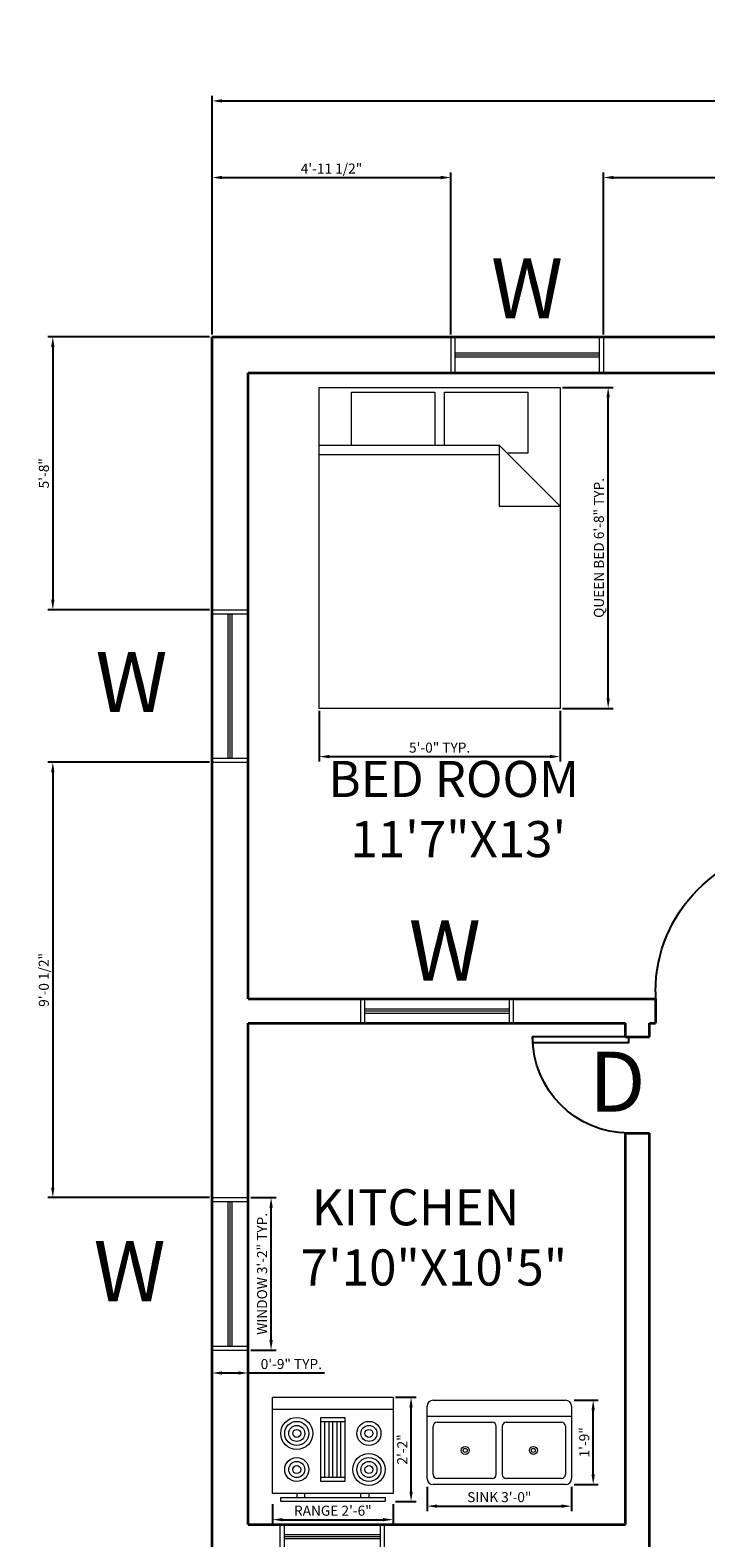
# Model space of a CAD drawing. Units: inches. Extents: x -8018 to -7514, y 7025 to 7863.
# Tile 2 of 3: x -8018 to -7850, y 7487 to 7863. Entities that reach past the tile are written whole.
import ezdxf

# ---------------------------------------------------------------- set-up
doc = ezdxf.new("R2010")
doc.units = ezdxf.units.IN
for name, color, linetype, lineweight, true_color in [('A-ANNO-DIMS', 30, 'Continuous', 18, 0xf26722), ('A-GLAZ', 240, 'Continuous', 18, 0xed1f24), ('A-WALL', 41, 'Continuous', 35, 0xf4ee51)]:
    doc.layers.add(name, color=color, linetype=linetype, lineweight=lineweight, true_color=true_color)
for name, color, linetype, lineweight in [('A-ANNO-TEXT', 7, 'Continuous', 18), ('A-AREA-IDEN', 7, 'Continuous', 18), ('A-DOOR', 4, 'Continuous', 25), ('A-EQPM', 9, 'Continuous', 18), ('A-FLOR-FIXT', 9, 'Continuous', 18), ('A-FURN', 9, 'Continuous', 18)]:
    doc.layers.add(name, color=color, linetype=linetype, lineweight=lineweight)
doc.styles.get("Standard").update_dxf_attribs({"font": 'arial.ttf'})
doc.dimstyles.new('ISO-25', dxfattribs={"dimtxt": 2.5, "dimasz": 2.5, "dimexe": 1.25, "dimexo": 0.625, "dimtad": 1, "dimdec": 0, "dimlunit": 3, "dimtxsty": 'Standard', "dimcen": 2.5, "dimadec": 0, "dimazin": 0, "dimtfac": 1, "dimtdec": 0, "dimtmove": 0, "dimatfit": 3, "dimfxl": 1, "dimarcsym": 0})

# ---------------------------------------------------------------- blocks, each defined once
blk = doc.blocks.new('*U8')
for p, q in [((0, 0), (0, -100)), ((750, 0), (750, -100))]:
    blk.add_line(p, q)
blk.add_lwpolyline([(0, 0), (0, 750), (43.75, 750), (43.75, 0)], close=True)
blk.add_arc((0, 0), 750, 0, 90)
blk = doc.blocks.new('Bed - Queen')
for p, q in [((0, -80.00003), (0, 0)), ((0, 0), (59.99999, 0)), ((59.99999, 0), (59.99999, -80.00003)), ((7.99999, -1.2), (28.79998, -1.2)), ((7.99999, -14.4), (7.99999, -1.2)), ((28.79998, -1.2), (28.79998, -14.4)), ((31.19999, -1.2), (51.99999, -1.2)), ((31.19999, -14.4), (31.19999, -1.2)), ((51.99999, -1.2), (51.99999, -16.4)), ((0, -14.4), (44.8, -14.4)), ((59.99999, -29.6), (44.8, -14.4)), ((44.8, -14.4), (44.8, -29.6)), ((44.8, -16.8), (0, -16.8)), ((51.99999, -16.4), (46.79936, -16.4)), ((44.8, -29.6), (59.99999, -29.6)), ((59.99999, -80.00003), (0, -80.00003))]:
    blk.add_line(p, q)
blk = doc.blocks.new('Range-Oven - 30 in top')
for p, q in [((0, -3), (30, -3)), ((12, -6), (18, -6)), ((13, -20), (13, -6)), ((14, -6), (14, -20)), ((15, -20), (15, -6)), ((16, -6), (16, -20)), ((17, -20), (17, -6)), ((18, -20), (12, -20)), ((6, -24), (6, -25)), ((8, -25), (8, -24)), ((22, -25), (22, -24)), ((24, -24), (24, -25))]:
    blk.add_line(p, q)
for points in [[(0, -24), (0, 0), (30, 0), (30, -24)], [(12, -21), (12, -5), (18, -5), (18, -21)], [(2, -26), (2, -25), (28, -25), (28, -26)]]:
    blk.add_lwpolyline(points, close=True)
for centre, radius in [((6, -9), 4), ((6, -9), 3), ((6, -9), 2), ((24, -9), 3), ((24, -9), 2), ((6, -9), 1), ((24, -9), 1), ((6, -18), 3), ((24, -18), 4), ((24, -18), 3), ((6, -18), 2), ((6, -18), 1), ((24, -18), 2), ((24, -18), 1)]:
    blk.add_circle(centre, radius)
blk = doc.blocks.new('Sink-double - 36 in top')
for p, q in [((-18, -4), (18, -4)), ((-0.75, -18.5), (-0.75, -6.5)), ((0.75, -6.5), (0.75, -18.5))]:
    blk.add_line(p, q)
for points in [[(-16.5, 0), (16.5, 0)], [(-18, -19.5), (-18, -1.5)], [(18, -1.5), (18, -19.5)], [(-16.5, -18.5), (-16.5, -6.5)], [(-15.5, -5.5), (-1.75, -5.5)], [(1.75, -5.5), (15.5, -5.5)], [(16.5, -6.5), (16.5, -18.5)], [(16.5, -21), (-16.5, -21)], [(-1.75, -19.5), (-15.5, -19.5)], [(15.5, -19.5), (1.75, -19.5)]]:
    blk.add_lwpolyline(points)
for centre, radius in [((-8.5, -12.5), 1), ((-8.5, -12.5), 0.5), ((8.5, -12.5), 1), ((8.5, -12.5), 0.5)]:
    blk.add_circle(centre, radius)
for centre, radius, start, end in [((-16.5, -1.5), 1.5, 90, 180), ((16.5, -1.5), 1.5, 0, 90), ((-15.5, -6.5), 1, 90, 180), ((-1.75, -6.5), 1, 0, 90), ((1.75, -6.5), 1, 90, 180), ((15.5, -6.5), 1, 0, 90), ((-15.5, -18.5), 1, 180, 270), ((-1.75, -18.5), 1, 270, 0), ((1.75, -18.5), 1, 180, 270), ((15.5, -18.5), 1, 270, 0), ((-16.5, -19.5), 1.5, 180, 270), ((16.5, -19.5), 1.5, 270, 0)]:
    blk.add_arc(centre, radius, start, end)
blk = doc.blocks.new('*D106')
at = {"layer": 'A-ANNO-DIMS', "color": 0, "lineweight": -2, "transparency": 16777216}
for p, q in [((-7972.8, 7786.99), (-7972.8, 7846.41)), ((-7970.3, 7845.16), (-7615.3, 7845.16)), ((-7612.8, 7786.99), (-7612.8, 7846.41))]:
    blk.add_line(p, q, dxfattribs=at)
at = {"layer": 'A-ANNO-DIMS', "color": 0, "transparency": 16777216}
for points in [[(-7970.3, 7845.58), (-7970.3, 7844.75), (-7972.8, 7845.16)], [(-7615.3, 7845.58), (-7615.3, 7844.75), (-7612.8, 7845.16)]]:
    blk.add_solid(points, dxfattribs=at)
at = {"layer": 'Defpoints', "color": 0, "transparency": 16777216}
for p in [(-7612.8, 7845.16), (-7972.8, 7786.37), (-7612.8, 7786.37)]:
    blk.add_point(p, dxfattribs=at)
at = {"layer": 'A-ANNO-DIMS', "color": 0, "transparency": 16777216, "insert": (-7792.8, 7853.96), "char_height": 2.5, "attachment_point": 5}
blk.add_mtext("{\\H6.4x;30'}", dxfattribs=at)
blk = doc.blocks.new('VENT-24IN-6IN-WALL')
for p, q in [((0, 26), (6, 26)), ((0, 25), (6, 25)), ((2.5, 1), (2.5, 25)), ((3, 1), (3, 25)), ((3.5, 1), (3.5, 25)), ((0, 1), (6, 1)), ((0, 0), (6, 0))]:
    blk.add_line(p, q)
blk = doc.blocks.new('WINDOW-36IN-6IN-WALL')
for p, q in [((0, 38), (6, 38)), ((0, 37), (6, 37)), ((2.5, 1), (2.5, 37)), ((3, 1), (3, 37)), ((3.5, 1), (3.5, 37)), ((0, 1), (6, 1)), ((0, 0), (6, 0))]:
    blk.add_line(p, q)
blk = doc.blocks.new('WINDOW-36IN-9IN-WALL-H')
for p, q in [((0, 9), (0, 0)), ((1, 9), (1, 0)), ((37, 9), (37, 0)), ((38, 9), (38, 0)), ((1, 5), (37, 5)), ((1, 4.5), (37, 4.5)), ((1, 4), (37, 4))]:
    blk.add_line(p, q)
blk = doc.blocks.new('WINDOW-36IN-9IN-WALL-V')
for p, q in [((0, 38), (9, 38)), ((0, 37), (9, 37)), ((4, 1), (4, 37)), ((4.5, 1), (4.5, 37)), ((5, 1), (5, 37)), ((0, 1), (9, 1)), ((0, 0), (9, 0))]:
    blk.add_line(p, q)
blk = doc.blocks.new('*D118')
at = {"layer": 'A-ANNO-DIMS', "color": 0, "lineweight": -2, "transparency": 16777216}
for p, q in [((-7963.17, 7571.87), (-7956.85, 7571.87)), ((-7958.1, 7536.37), (-7958.1, 7569.37)), ((-7963.17, 7533.87), (-7956.85, 7533.87))]:
    blk.add_line(p, q, dxfattribs=at)
at = {"layer": 'A-ANNO-DIMS', "color": 0, "transparency": 16777216}
for points in [[(-7958.52, 7569.37), (-7957.68, 7569.37), (-7958.1, 7571.87)], [(-7958.52, 7536.37), (-7957.68, 7536.37), (-7958.1, 7533.87)]]:
    blk.add_solid(points, dxfattribs=at)
at = {"layer": 'Defpoints', "color": 0, "transparency": 16777216}
for p in [(-7963.8, 7571.87), (-7958.1, 7571.87), (-7963.8, 7533.87)]:
    blk.add_point(p, dxfattribs=at)
at = {"layer": 'A-ANNO-DIMS', "color": 0, "transparency": 16777216, "insert": (-7960.02, 7552.87), "char_height": 2.5, "attachment_point": 5, "rotation": 90}
blk.add_mtext('WINDOW 3\'-2" TYP.', dxfattribs=at)
blk = doc.blocks.new('*D119')
at = {"layer": 'A-ANNO-DIMS', "color": 0, "lineweight": -2, "transparency": 16777216}
for p, q in [((-7972.8, 7533.24), (-7972.8, 7526.92)), ((-7963.8, 7533.24), (-7963.8, 7526.92)), ((-7970.3, 7528.17), (-7966.3, 7528.17)), ((-7963.8, 7528.17), (-7944.81, 7528.17))]:
    blk.add_line(p, q, dxfattribs=at)
at = {"layer": 'A-ANNO-DIMS', "color": 0, "transparency": 16777216}
for points in [[(-7970.3, 7528.58), (-7970.3, 7527.75), (-7972.8, 7528.17)], [(-7966.3, 7528.58), (-7966.3, 7527.75), (-7963.8, 7528.17)]]:
    blk.add_solid(points, dxfattribs=at)
at = {"layer": 'Defpoints', "color": 0, "transparency": 16777216}
for p in [(-7972.8, 7533.87), (-7963.8, 7533.87), (-7963.8, 7528.17)]:
    blk.add_point(p, dxfattribs=at)
at = {"layer": 'A-ANNO-DIMS', "color": 0, "transparency": 16777216, "insert": (-7953.06, 7530.07), "char_height": 2.5, "attachment_point": 5}
blk.add_mtext('0\'-9" TYP.', dxfattribs=at)
blk = doc.blocks.new('*D122')
at = {"layer": 'A-ANNO-DIMS', "color": 0, "lineweight": -2, "transparency": 16777216}
for p, q in [((-7885.47, 7773.77), (-7872.85, 7773.77)), ((-7874.1, 7696.27), (-7874.1, 7771.27)), ((-7885.47, 7693.77), (-7872.85, 7693.77))]:
    blk.add_line(p, q, dxfattribs=at)
at = {"layer": 'A-ANNO-DIMS', "color": 0, "transparency": 16777216}
for points in [[(-7874.51, 7771.27), (-7873.68, 7771.27), (-7874.1, 7773.77)], [(-7874.51, 7696.27), (-7873.68, 7696.27), (-7874.1, 7693.77)]]:
    blk.add_solid(points, dxfattribs=at)
at = {"layer": 'Defpoints', "color": 0, "transparency": 16777216}
for p in [(-7886.1, 7773.77), (-7874.1, 7773.77), (-7886.1, 7693.77)]:
    blk.add_point(p, dxfattribs=at)
at = {"layer": 'A-ANNO-DIMS', "color": 0, "transparency": 16777216, "insert": (-7876.09, 7733.77), "char_height": 2.5, "attachment_point": 5, "rotation": 90}
blk.add_mtext('QUEEN BED 6\'-8" TYP.', dxfattribs=at)
blk = doc.blocks.new('*D123')
at = {"layer": 'A-ANNO-DIMS', "color": 0, "lineweight": -2, "transparency": 16777216}
for p, q in [((-7946.1, 7693.15), (-7946.1, 7680.52)), ((-7886.1, 7693.15), (-7886.1, 7680.52)), ((-7943.6, 7681.77), (-7888.6, 7681.77))]:
    blk.add_line(p, q, dxfattribs=at)
at = {"layer": 'A-ANNO-DIMS', "color": 0, "transparency": 16777216}
for points in [[(-7943.6, 7682.19), (-7943.6, 7681.35), (-7946.1, 7681.77)], [(-7888.6, 7682.19), (-7888.6, 7681.35), (-7886.1, 7681.77)]]:
    blk.add_solid(points, dxfattribs=at)
at = {"layer": 'Defpoints', "color": 0, "transparency": 16777216}
for p in [(-7946.1, 7693.77), (-7886.1, 7693.77), (-7886.1, 7681.77)]:
    blk.add_point(p, dxfattribs=at)
at = {"layer": 'A-ANNO-DIMS', "color": 0, "transparency": 16777216, "insert": (-7916.1, 7683.67), "char_height": 2.5, "attachment_point": 5}
blk.add_mtext('5\'-0" TYP.', dxfattribs=at)
blk = doc.blocks.new('*D124')
at = {"layer": 'A-ANNO-DIMS', "color": 0, "lineweight": -2, "transparency": 16777216}
for p, q in [((-7957.71, 7495.48), (-7957.71, 7490.36)), ((-7927.71, 7495.48), (-7927.71, 7490.36)), ((-7955.21, 7491.61), (-7930.21, 7491.61))]:
    blk.add_line(p, q, dxfattribs=at)
at = {"layer": 'A-ANNO-DIMS', "color": 0, "transparency": 16777216}
for points in [[(-7955.21, 7492.02), (-7955.21, 7491.19), (-7957.71, 7491.61)], [(-7930.21, 7492.02), (-7930.21, 7491.19), (-7927.71, 7491.61)]]:
    blk.add_solid(points, dxfattribs=at)
at = {"layer": 'Defpoints', "color": 0, "transparency": 16777216}
for p in [(-7957.71, 7496.11), (-7927.71, 7496.11), (-7927.71, 7491.61)]:
    blk.add_point(p, dxfattribs=at)
at = {"layer": 'A-ANNO-DIMS', "color": 0, "transparency": 16777216, "insert": (-7942.71, 7493.53), "char_height": 2.5, "attachment_point": 5}
blk.add_mtext('RANGE 2\'-6"', dxfattribs=at)
blk = doc.blocks.new('*D125')
at = {"layer": 'A-ANNO-DIMS', "color": 0, "lineweight": -2, "transparency": 16777216}
for p, q in [((-7927.09, 7522.11), (-7921.96, 7522.11)), ((-7923.21, 7498.61), (-7923.21, 7519.61)), ((-7927.09, 7496.11), (-7921.96, 7496.11))]:
    blk.add_line(p, q, dxfattribs=at)
at = {"layer": 'A-ANNO-DIMS', "color": 0, "transparency": 16777216}
for points in [[(-7923.63, 7519.61), (-7922.8, 7519.61), (-7923.21, 7522.11)], [(-7923.63, 7498.61), (-7922.8, 7498.61), (-7923.21, 7496.11)]]:
    blk.add_solid(points, dxfattribs=at)
at = {"layer": 'Defpoints', "color": 0, "transparency": 16777216}
for p in [(-7927.71, 7522.11), (-7923.21, 7522.11), (-7927.71, 7496.11)]:
    blk.add_point(p, dxfattribs=at)
at = {"layer": 'A-ANNO-DIMS', "color": 0, "transparency": 16777216, "insert": (-7925.09, 7509.11), "char_height": 2.5, "attachment_point": 5, "rotation": 90}
blk.add_mtext('2\'-2"', dxfattribs=at)
blk = doc.blocks.new('*D126')
at = {"layer": 'A-ANNO-DIMS', "color": 0, "lineweight": -2, "transparency": 16777216}
for p, q in [((-7919.23, 7499.76), (-7919.23, 7493.73)), ((-7883.23, 7499.76), (-7883.23, 7493.73)), ((-7916.73, 7494.98), (-7885.73, 7494.98))]:
    blk.add_line(p, q, dxfattribs=at)
at = {"layer": 'A-ANNO-DIMS', "color": 0, "transparency": 16777216}
for points in [[(-7916.73, 7495.4), (-7916.73, 7494.57), (-7919.23, 7494.98)], [(-7885.73, 7495.4), (-7885.73, 7494.57), (-7883.23, 7494.98)]]:
    blk.add_solid(points, dxfattribs=at)
at = {"layer": 'Defpoints', "color": 0, "transparency": 16777216}
for p in [(-7919.23, 7500.38), (-7883.23, 7500.38), (-7883.23, 7494.98)]:
    blk.add_point(p, dxfattribs=at)
at = {"layer": 'A-ANNO-DIMS', "color": 0, "transparency": 16777216, "insert": (-7901.23, 7496.9), "char_height": 2.5, "attachment_point": 5}
blk.add_mtext('SINK 3\'-0"', dxfattribs=at)
blk = doc.blocks.new('*D127')
at = {"layer": 'A-ANNO-DIMS', "color": 0, "lineweight": -2, "transparency": 16777216}
for p, q in [((-7882.61, 7521.38), (-7876.58, 7521.38)), ((-7877.83, 7502.88), (-7877.83, 7518.88)), ((-7882.61, 7500.38), (-7876.58, 7500.38))]:
    blk.add_line(p, q, dxfattribs=at)
at = {"layer": 'A-ANNO-DIMS', "color": 0, "transparency": 16777216}
for points in [[(-7878.25, 7518.88), (-7877.42, 7518.88), (-7877.83, 7521.38)], [(-7878.25, 7502.88), (-7877.42, 7502.88), (-7877.83, 7500.38)]]:
    blk.add_solid(points, dxfattribs=at)
at = {"layer": 'Defpoints', "color": 0, "transparency": 16777216}
for p in [(-7883.23, 7521.38), (-7877.83, 7521.38), (-7883.23, 7500.38)]:
    blk.add_point(p, dxfattribs=at)
at = {"layer": 'A-ANNO-DIMS', "color": 0, "transparency": 16777216, "insert": (-7879.73, 7510.88), "char_height": 2.5, "attachment_point": 5, "rotation": 90}
blk.add_mtext('1\'-9"', dxfattribs=at)
blk = doc.blocks.new('*D138')
at = {"layer": 'A-ANNO-DIMS', "color": 0, "lineweight": -2, "transparency": 16777216}
for p, q in [((-7972.8, 7786.99), (-7972.8, 7827.32)), ((-7970.3, 7826.07), (-7915.8, 7826.07)), ((-7913.3, 7786.99), (-7913.3, 7827.32))]:
    blk.add_line(p, q, dxfattribs=at)
at = {"layer": 'A-ANNO-DIMS', "color": 0, "transparency": 16777216}
for points in [[(-7970.3, 7826.48), (-7970.3, 7825.65), (-7972.8, 7826.07)], [(-7915.8, 7826.48), (-7915.8, 7825.65), (-7913.3, 7826.07)]]:
    blk.add_solid(points, dxfattribs=at)
at = {"layer": 'Defpoints', "color": 0, "transparency": 16777216}
for p in [(-7913.3, 7826.07), (-7972.8, 7786.37), (-7913.3, 7786.37)]:
    blk.add_point(p, dxfattribs=at)
at = {"layer": 'A-ANNO-DIMS', "color": 0, "transparency": 16777216, "insert": (-7943.05, 7827.98), "char_height": 2.5, "attachment_point": 5}
blk.add_mtext('4\'-11 1/2"', dxfattribs=at)
blk = doc.blocks.new('*D139')
at = {"layer": 'A-ANNO-DIMS', "color": 0, "lineweight": -2, "transparency": 16777216}
for p, q in [((-7875.3, 7786.99), (-7875.3, 7827.32)), ((-7872.8, 7826.07), (-7767.8, 7826.07)), ((-7765.3, 7786.99), (-7765.3, 7827.32))]:
    blk.add_line(p, q, dxfattribs=at)
at = {"layer": 'A-ANNO-DIMS', "color": 0, "transparency": 16777216}
for points in [[(-7872.8, 7826.48), (-7872.8, 7825.65), (-7875.3, 7826.07)], [(-7767.8, 7826.48), (-7767.8, 7825.65), (-7765.3, 7826.07)]]:
    blk.add_solid(points, dxfattribs=at)
at = {"layer": 'Defpoints', "color": 0, "transparency": 16777216}
for p in [(-7765.3, 7826.07), (-7875.3, 7786.37), (-7765.3, 7786.37)]:
    blk.add_point(p, dxfattribs=at)
at = {"layer": 'A-ANNO-DIMS', "color": 0, "transparency": 16777216, "insert": (-7820.3, 7827.97), "char_height": 2.5, "attachment_point": 5}
blk.add_mtext('9\'-2"', dxfattribs=at)
blk = doc.blocks.new('*D140')
at = {"layer": 'A-ANNO-DIMS', "color": 0, "lineweight": -2, "transparency": 16777216}
for p, q in [((-7973.42, 7786.37), (-8013.75, 7786.37)), ((-8012.5, 7783.87), (-8012.5, 7720.87)), ((-7973.42, 7718.37), (-8013.75, 7718.37))]:
    blk.add_line(p, q, dxfattribs=at)
at = {"layer": 'A-ANNO-DIMS', "color": 0, "transparency": 16777216}
for points in [[(-8012.92, 7783.87), (-8012.08, 7783.87), (-8012.5, 7786.37)], [(-8012.92, 7720.87), (-8012.08, 7720.87), (-8012.5, 7718.37)]]:
    blk.add_solid(points, dxfattribs=at)
at = {"layer": 'Defpoints', "color": 0, "transparency": 16777216}
for p in [(-7972.8, 7786.37), (-8012.5, 7718.37), (-7972.8, 7718.37)]:
    blk.add_point(p, dxfattribs=at)
at = {"layer": 'A-ANNO-DIMS', "color": 0, "transparency": 16777216, "insert": (-8014.4, 7752.37), "char_height": 2.5, "attachment_point": 5, "rotation": 90}
blk.add_mtext('5\'-8"', dxfattribs=at)
blk = doc.blocks.new('*D141')
at = {"layer": 'A-ANNO-DIMS', "color": 0, "lineweight": -2, "transparency": 16777216}
for p, q in [((-7973.42, 7680.37), (-8013.75, 7680.37)), ((-8012.5, 7677.87), (-8012.5, 7574.37)), ((-7973.42, 7571.87), (-8013.75, 7571.87))]:
    blk.add_line(p, q, dxfattribs=at)
at = {"layer": 'A-ANNO-DIMS', "color": 0, "transparency": 16777216}
for points in [[(-8012.92, 7677.87), (-8012.08, 7677.87), (-8012.5, 7680.37)], [(-8012.92, 7574.37), (-8012.08, 7574.37), (-8012.5, 7571.87)]]:
    blk.add_solid(points, dxfattribs=at)
at = {"layer": 'Defpoints', "color": 0, "transparency": 16777216}
for p in [(-7972.8, 7680.37), (-8012.5, 7571.87), (-7972.8, 7571.87)]:
    blk.add_point(p, dxfattribs=at)
at = {"layer": 'A-ANNO-DIMS', "color": 0, "transparency": 16777216, "insert": (-8014.42, 7626.12), "char_height": 2.5, "attachment_point": 5, "rotation": 90}
blk.add_mtext('9\'-0 1/2"', dxfattribs=at)

msp = doc.modelspace()

# ---------------------------------------------------------------- linework, layer by layer
at = {"layer": 'A-WALL'}
for p, q in [((-7972.8, 7786.37), (-7612.8, 7786.37)), ((-7972.8, 7066.37), (-7972.8, 7786.37)), ((-7963.8, 7777.37), (-7824.8, 7777.37)), ((-7963.8, 7621.37), (-7963.8, 7777.37)), ((-7963.8, 7621.37), (-7862.3, 7621.37)), ((-7862.3, 7621.37), (-7862.3, 7615.37)), ((-7963.8, 7615.37), (-7869.8, 7615.37)), ((-7963.8, 7490.37), (-7963.8, 7615.37)), ((-7869.8, 7611.95), (-7869.8, 7615.37)), ((-7869.8, 7611.95), (-7863.8, 7611.95)), ((-7863.8, 7615.37), (-7862.3, 7615.37)), ((-7863.8, 7611.95), (-7863.8, 7615.37)), ((-7869.8, 7490.37), (-7869.8, 7587.95)), ((-7869.8, 7587.95), (-7863.8, 7587.95)), ((-7863.8, 7484.37), (-7863.8, 7587.95)), ((-7963.8, 7490.37), (-7869.8, 7490.37))]:
    msp.add_line(p, q, dxfattribs=at)

# ---------------------------------------------------------------- block references
at = {"layer": 'A-DOOR', "xscale": -0.0480000071715659, "yscale": 0.0480000071715659, "zscale": 0.0480000071715659}
msp.add_blockref('*U8', (-7826.3, 7623.17), dxfattribs=at)
at = {"layer": 'A-DOOR', "xscale": -0.0319973580388838, "yscale": 0.0319973580388838, "zscale": 0.0319973580388838, "rotation": 90}
msp.add_blockref('*U8', (-7868.95, 7611.95), dxfattribs=at)
at = {"layer": 'A-EQPM'}
msp.add_blockref('Range-Oven - 30 in top', (-7957.71, 7522.11), dxfattribs=at)
at = {"layer": 'A-FLOR-FIXT'}
msp.add_blockref('Sink-double - 36 in top', (-7901.23, 7521.38), dxfattribs=at)
at = {"layer": 'A-FURN'}
msp.add_blockref('Bed - Queen', (-7946.1, 7773.77), dxfattribs=at)
at = {"layer": 'A-GLAZ'}
for name, p in [('WINDOW-36IN-9IN-WALL-H', (-7913.3, 7777.37)), ('WINDOW-36IN-9IN-WALL-V', (-7972.8, 7680.37)), ('WINDOW-36IN-9IN-WALL-V', (-7972.8, 7533.87))]:
    msp.add_blockref(name, p, dxfattribs=at)
for name, p, rotation in [('WINDOW-36IN-6IN-WALL', (-7935.8, 7621.37), 270.0000000000103), ('VENT-24IN-6IN-WALL', (-7929.8, 7484.37), 89.99999999999126)]:
    msp.add_blockref(name, p, dxfattribs=dict(at, rotation=rotation))

# ---------------------------------------------------------------- texts
at = {"layer": 'A-ANNO-TEXT', "char_height": 15, "attachment_point": 1}
for s, insert in [('{W}', (-7903.3, 7805.95)), ('{W}', (-8001.87, 7707.84)), ('{W}', (-7923.79, 7640.95)), ('{D}', (-7878.86, 7608.25)), ('{W}', (-8002.34, 7561.06))]:
    msp.add_mtext_dynamic_manual_height_columns(s, width=548.1497, gutter_width=12.5, heights=[0], dxfattribs=dict(at, insert=insert))
at = {"layer": 'A-AREA-IDEN', "char_height": 9, "attachment_point": 1}
for s, insert in [('{BED ROOM\\P  11\'7"X13\'}', (-7943.83, 7680.7)), ('{ KITCHEN\\P7\'10"X10\'5"}', (-7950.72, 7573.96))]:
    msp.add_mtext_dynamic_manual_height_columns(s, width=697.6004, gutter_width=12.5, heights=[0], dxfattribs=dict(at, insert=insert))

# ---------------------------------------------------------------- dimensions: what is measured, and where the dimension line sits
at = {"layer": 'A-ANNO-DIMS'}
for base, p1, p2, text, override, picture, middle in [((-7612.8, 7845.16), (-7972.8, 7786.37), (-7612.8, 7786.37), '{\\H6.4x;<>}', {"dimclrd": 0, "dimclre": 0, "dimclrt": 0}, '*D106', (-7792.8, 7853.96)), ((-7886.1, 7681.77), (-7946.1, 7693.77), (-7886.1, 7693.77), '<> TYP.', {"dimdec": 1, "dimlfac": 1, "dimrnd": 0, "dimzin": 1, "dimdsep": 46, "dimlunit": 4, "dimfrac": 2}, '*D123', (-7916.1, 7683.67)), ((-7963.8, 7528.17), (-7972.8, 7533.87), (-7963.8, 7533.87), '<> TYP.', {"dimdec": 1, "dimlfac": 1, "dimrnd": 0, "dimzin": 1, "dimdsep": 46, "dimlunit": 4, "dimfrac": 2}, '*D119', (-7953.06, 7530.07)), ((-7883.23, 7494.98), (-7919.23, 7500.38), (-7883.23, 7500.38), 'SINK <>', {"dimdec": 1, "dimlfac": 1, "dimrnd": 0, "dimzin": 1, "dimdsep": 46, "dimlunit": 4, "dimfrac": 2}, '*D126', (-7901.23, 7496.9)), ((-7927.71, 7491.61), (-7957.71, 7496.11), (-7927.71, 7496.11), 'RANGE <>', {"dimdec": 1, "dimlfac": 1, "dimrnd": 0, "dimzin": 1, "dimdsep": 46, "dimlunit": 4, "dimfrac": 2}, '*D124', (-7942.71, 7493.53))]:
    dim = msp.add_linear_dim(base=base, p1=p1, p2=p2, text=text, dimstyle='ISO-25', override=override, dxfattribs=at)
    dim.commit()
    dim.dimension.update_dxf_attribs({"geometry": picture, "text_midpoint": middle})
for base, p1, p2, picture, middle in [((-7913.3, 7826.07), (-7972.8, 7786.37), (-7913.3, 7786.37), '*D138', (-7943.05, 7827.98)), ((-7765.3, 7826.07), (-7875.3, 7786.37), (-7765.3, 7786.37), '*D139', (-7820.3, 7827.97))]:
    dim = msp.add_linear_dim(base=base, p1=p1, p2=p2, dimstyle='ISO-25', override={"dimdec": 1, "dimlfac": 1, "dimrnd": 0, "dimzin": 1, "dimdsep": 46, "dimlunit": 4, "dimfrac": 2}, dxfattribs=at)
    dim.commit()
    dim.dimension.update_dxf_attribs({"geometry": picture, "text_midpoint": middle})
for base, p1, p2, picture, middle in [((-8012.5, 7718.37), (-7972.8, 7786.37), (-7972.8, 7718.37), '*D140', (-8014.4, 7752.37)), ((-8012.5, 7571.87), (-7972.8, 7680.37), (-7972.8, 7571.87), '*D141', (-8014.42, 7626.12)), ((-7923.21, 7522.11), (-7927.71, 7496.11), (-7927.71, 7522.11), '*D125', (-7925.09, 7509.11)), ((-7877.83, 7521.38), (-7883.23, 7500.38), (-7883.23, 7521.38), '*D127', (-7879.73, 7510.88))]:
    dim = msp.add_linear_dim(base=base, p1=p1, p2=p2, angle=90, dimstyle='ISO-25', override={"dimdec": 1, "dimlfac": 1, "dimrnd": 0, "dimzin": 1, "dimdsep": 46, "dimlunit": 4, "dimfrac": 2}, dxfattribs=at)
    dim.commit()
    dim.dimension.update_dxf_attribs({"geometry": picture, "text_midpoint": middle})
for base, p1, p2, text, picture, middle in [((-7874.1, 7773.77), (-7886.1, 7693.77), (-7886.1, 7773.77), 'QUEEN BED <> TYP.', '*D122', (-7876.09, 7733.77)), ((-7958.1, 7571.87), (-7963.8, 7533.87), (-7963.8, 7571.87), 'WINDOW <> TYP.', '*D118', (-7960.02, 7552.87))]:
    dim = msp.add_linear_dim(base=base, p1=p1, p2=p2, angle=90, text=text, dimstyle='ISO-25', override={"dimdec": 1, "dimlfac": 1, "dimrnd": 0, "dimzin": 1, "dimdsep": 46, "dimlunit": 4, "dimfrac": 2}, dxfattribs=at)
    dim.commit()
    dim.dimension.update_dxf_attribs({"geometry": picture, "text_midpoint": middle})

doc.saveas('drawing.dxf')
